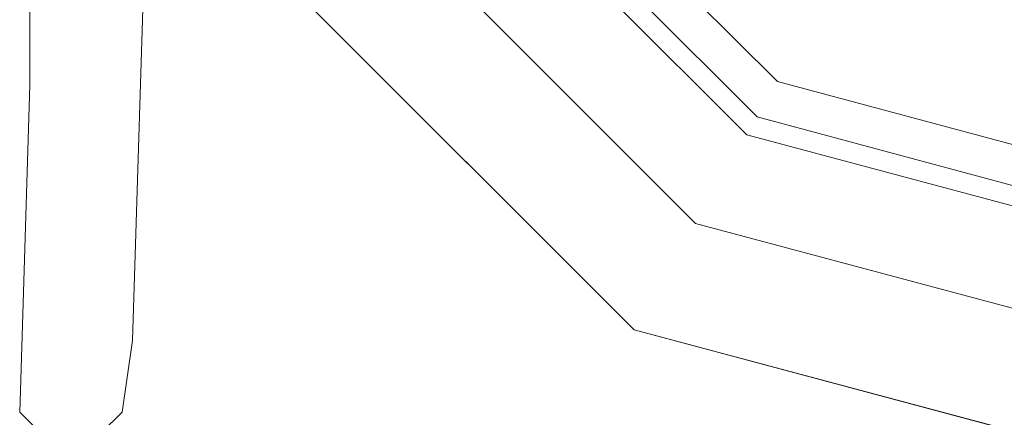
# Model space of a CAD drawing. Units: inches. Extents: x 375 to 1122, y 27 to 1069.
# Tile 52 of 155: x 719.619 to 725.537, y 311.85 to 314.242. Entities that reach past the tile are written whole.
import ezdxf

# ---------------------------------------------------------------- set-up
doc = ezdxf.new("R2010")
doc.units = ezdxf.units.IN
doc.layers.add('Furniture', color=30, linetype='Continuous', lineweight=18)

# ---------------------------------------------------------------- blocks, each defined once
blk = doc.blocks.new('A$C403C54AD')
at = {"linetype": 'ByBlock', "invisible_edges": 5}
for points in [[(0.81594, 0.97759, -0.02585), (0.72796, 1.02838, -0.02585), (0.72796, 1.02838, -0.02585), (0.82955, 1.02838, -0.02585)], [(0.77876, 0.94041, -0.02585), (0.72796, 1.02838, -0.02585), (0.72796, 1.02838, -0.02585), (0.81594, 0.97759, -0.02585)], [(0.81061, 0.98067, -0.04278), (0.81861, 0.97605, -0.03355), (0.83263, 1.02838, -0.03355), (0.82339, 1.02838, -0.04278)], [(0.83194, 0.96835, -0.0197), (0.81594, 0.97759, -0.02585), (0.82955, 1.02838, -0.02585), (0.84802, 1.02838, -0.0197)], [(0.81861, 0.97605, -0.03355), (0.84793, 0.95912, -0.02431), (0.86649, 1.02838, -0.02431), (0.83263, 1.02838, -0.03355)], [(0.84793, 0.95912, -0.0197), (0.83194, 0.96835, -0.0197), (0.84802, 1.02838, -0.0197), (0.86649, 1.02838, -0.0197)], [(0.77568, 0.94574, -0.04278), (0.7803, 0.93774, -0.03355), (0.81861, 0.97605, -0.03355), (0.81061, 0.98067, -0.04278)], [(0.78799, 0.92441, -0.0197), (0.77876, 0.94041, -0.02585), (0.81594, 0.97759, -0.02585), (0.83194, 0.96835, -0.0197)], [(0.7803, 0.93774, -0.03355), (0.79723, 0.90841, -0.02431), (0.84793, 0.95912, -0.02431), (0.81861, 0.97605, -0.03355)], [(0.79723, 0.90841, -0.0197), (0.78799, 0.92441, -0.0197), (0.83194, 0.96835, -0.0197), (0.84793, 0.95912, -0.0197)]]:
    blk.add_3dface(points, dxfattribs=at)
at = {"linetype": 'ByBlock'}
for points in [[(0.84793, 0.95912, -0.02431), (0.84793, 0.95912, -0.0197), (0.86649, 1.02838, -0.0197), (0.86649, 1.02838, -0.02431)], [(0.79723, 0.90841, -0.02431), (0.79723, 0.90841, -0.0197), (0.84793, 0.95912, -0.0197), (0.84793, 0.95912, -0.02431)]]:
    blk.add_3dface(points, dxfattribs=at)
at = {"invisible_edges": 5}
for points in [[(0.81108, 0.86831, -0.03586), (0.84956, 0.8837, -0.03586), (0.75259, 0.88678, -0.03586), (0.75259, 0.86831, -0.03586)], [(0.81108, 0.86831, -0.0374), (0.84956, 0.8837, -0.0374), (0.75259, 0.88678, -0.0374), (0.75259, 0.86831, -0.0374)], [(0.84956, 0.8837, -0.0374), (0.84956, 0.8837, -0.03586), (0.75259, 0.88678, -0.03586), (0.75259, 0.88678, -0.0374)], [(0.86033, 0.88216, -0.03586), (0.86033, 0.86677, -0.03586), (0.81108, 0.86831, -0.03586), (0.84956, 0.8837, -0.03586)], [(0.86033, 0.88216, -0.0374), (0.86033, 0.86677, -0.0374), (0.81108, 0.86831, -0.0374), (0.84956, 0.8837, -0.0374)], [(0.86033, 0.88216, -0.03586), (0.86033, 0.88216, -0.0374), (0.84956, 0.8837, -0.0374), (0.84956, 0.8837, -0.03586)], [(0.86341, 0.86985, -0.03586), (0.86341, 0.87908, -0.03586), (0.86033, 0.88216, -0.03586), (0.86033, 0.86677, -0.03586)], [(0.86341, 0.86985, -0.0374), (0.86341, 0.87908, -0.0374), (0.86033, 0.88216, -0.0374), (0.86033, 0.86677, -0.0374)], [(0.86341, 0.87908, -0.0374), (0.86341, 0.87908, -0.03586), (0.86033, 0.88216, -0.03586), (0.86033, 0.88216, -0.0374)], [(0.86033, 0.86677, -0.03586), (0.86033, 0.86677, -0.0374), (0.86341, 0.86985, -0.0374), (0.86341, 0.86985, -0.03586)], [(0.75259, 0.86831, -0.03586), (0.75259, 0.86831, -0.0374), (0.81108, 0.86831, -0.0374), (0.81108, 0.86831, -0.03586)], [(0.81108, 0.86831, -0.0374), (0.81108, 0.86831, -0.03586), (0.86033, 0.86677, -0.03586), (0.86033, 0.86677, -0.0374)]]:
    blk.add_3dface(points, dxfattribs=at)

msp = doc.modelspace()

# ---------------------------------------------------------------- block references
at = {"layer": 'Furniture', "xscale": 39.9918517141215, "yscale": 39.9918517141215, "zscale": 39.9918517141215, "rotation": 270}
msp.add_blockref('A$C403C54AD', (684.9549, 346.2875, 0.024), dxfattribs=at)

doc.saveas('drawing.dxf')
